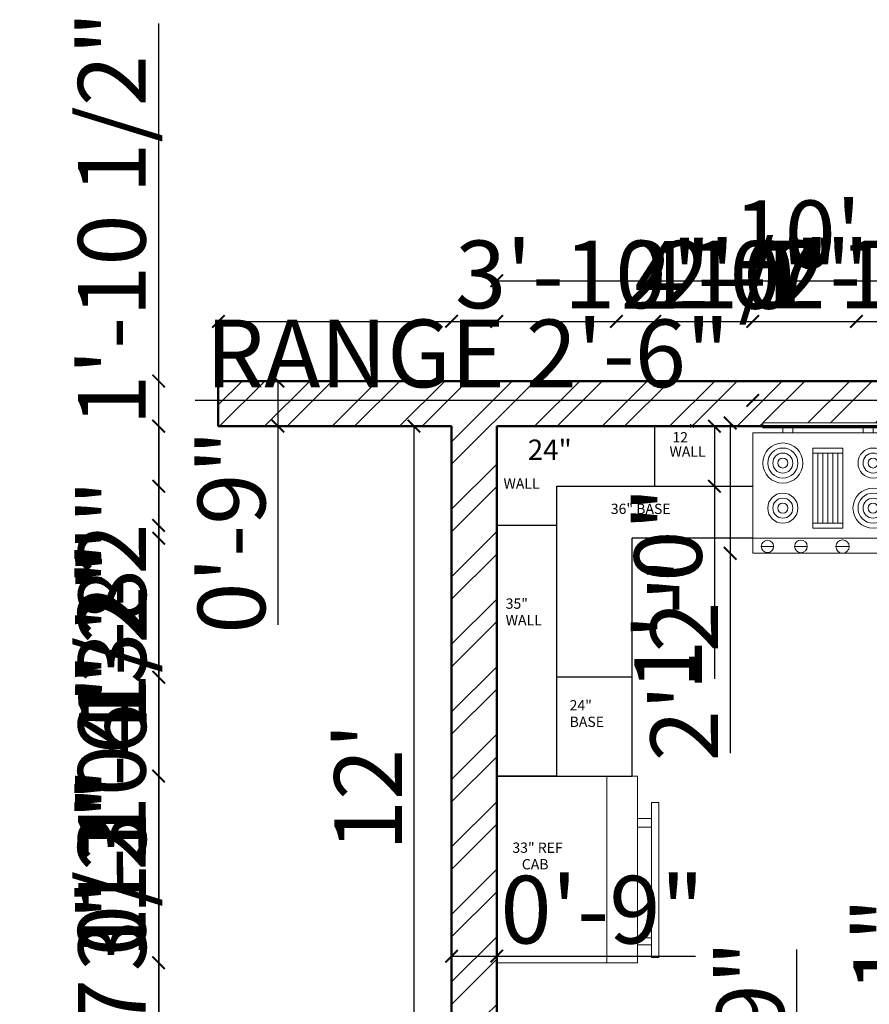
# Model space of a CAD drawing. Units: inches. Extents: x 1736 to 2023, y 1717 to 2014.
# Tile 2 of 3: x 1736 to 1906, y 1818 to 2014. Entities that reach past the tile are written whole.
import ezdxf

# ---------------------------------------------------------------- set-up
doc = ezdxf.new("R2010")
doc.units = ezdxf.units.IN
for name, color, linetype, lineweight in [('A-ANNO-DIMS', 2, 'Continuous', 18), ('A-ANNO-TEXT', 3, 'Continuous', 18), ('A-EQPM', 9, 'Continuous', 18), ('A-FLOR-CASE', 8, 'Continuous', 25), ('A-WALL', 7, 'Continuous', 50), ('A-WALL-PATT', 8, 'Continuous', 13)]:
    doc.layers.add(name, color=color, linetype=linetype, lineweight=lineweight)
doc.styles.get("Standard").update_dxf_attribs({"font": 'arial.ttf'})
doc.dimstyles.new('ISO-25', dxfattribs={"dimtxt": 13.5, "dimasz": 2.5, "dimexe": 1.25, "dimexo": 0.625, "dimtad": 1, "dimdec": 0, "dimlunit": 4, "dimtxsty": 'Standard', "dimblk": 'ARCHTICK', "dimcen": 2.5, "dimse1": 1, "dimse2": 1, "dimclrd": 2, "dimclrt": 4, "dimadec": 0, "dimazin": 0, "dimtfac": 1, "dimtdec": 0, "dimtmove": 0, "dimatfit": 3, "dimfxl": 1, "dimarcsym": 0})

# ---------------------------------------------------------------- blocks, each defined once
blk = doc.blocks.new('Range-Oven - 30 in top')
for p, q in [((0, -3), (30, -3)), ((12, -6), (18, -6)), ((13, -20), (13, -6)), ((14, -6), (14, -20)), ((15, -20), (15, -6)), ((16, -6), (16, -20)), ((17, -20), (17, -6)), ((18, -20), (12, -20)), ((6, -24), (6, -25)), ((8, -25), (8, -24)), ((22, -25), (22, -24)), ((24, -24), (24, -25))]:
    blk.add_line(p, q)
for points in [[(0, -24), (0, 0), (30, 0), (30, -24)], [(12, -21), (12, -5), (18, -5), (18, -21)], [(2, -26), (2, -25), (28, -25), (28, -26)]]:
    blk.add_lwpolyline(points, close=True)
for centre, radius in [((6, -9), 4), ((6, -9), 3), ((6, -9), 2), ((24, -9), 3), ((24, -9), 2), ((6, -9), 1), ((24, -9), 1), ((6, -18), 3), ((24, -18), 4), ((24, -18), 3), ((6, -18), 2), ((6, -18), 1), ((24, -18), 2), ((24, -18), 1)]:
    blk.add_circle(centre, radius)
blk = doc.blocks.new('_ArchTick')
at = {"color": 0, "linetype": 'ByBlock', "const_width": 0.15}
blk.add_lwpolyline([(-0.5, -0.5), (0.5, 0.5)], dxfattribs=at)
blk = doc.blocks.new('*D7')
at = {"layer": 'A-ANNO-DIMS', "color": 0, "lineweight": -2, "transparency": 16777216}
blk.add_line((1831.43, 1962.29), (1951.43, 1962.29), dxfattribs=at)
at = {"layer": 'Defpoints', "color": 0, "transparency": 16777216}
for p in [(1951.43, 1962.29), (1831.43, 1933.29), (1951.43, 1933.29)]:
    blk.add_point(p, dxfattribs=at)
at = {"layer": 'A-ANNO-DIMS', "color": 0, "lineweight": -2, "transparency": 16777216, "xscale": 2.5, "yscale": 2.5, "zscale": 2.5, "rotation": 180}
blk.add_blockref('_ArchTick', (1831.43, 1962.29), dxfattribs=at)
at = {"layer": 'A-ANNO-DIMS', "color": 0, "lineweight": -2, "transparency": 16777216, "xscale": 2.5, "yscale": 2.5, "zscale": 2.5}
blk.add_blockref('_ArchTick', (1951.43, 1962.29), dxfattribs=at)
at = {"layer": 'A-ANNO-DIMS', "color": 0, "transparency": 16777216, "insert": (1891.43, 1969.8), "char_height": 13.5, "attachment_point": 5}
blk.add_mtext("10'", dxfattribs=at)
blk = doc.blocks.new('*D8')
at = {"layer": 'A-ANNO-DIMS', "color": 0, "lineweight": -2, "transparency": 16777216}
blk.add_line((1814.91, 1933.29), (1814.91, 1789.29), dxfattribs=at)
at = {"layer": 'Defpoints', "color": 0, "transparency": 16777216}
for p in [(1822.43, 1933.29), (1814.91, 1789.29), (1822.43, 1789.29)]:
    blk.add_point(p, dxfattribs=at)
at = {"layer": 'A-ANNO-DIMS', "color": 0, "lineweight": -2, "transparency": 16777216, "xscale": 2.5, "yscale": 2.5, "zscale": 2.5}
for p, rotation in [((1814.91, 1933.29), 90), ((1814.91, 1789.29), 270)]:
    blk.add_blockref('_ArchTick', p, dxfattribs=dict(at, rotation=rotation))
at = {"layer": 'A-ANNO-DIMS', "color": 0, "transparency": 16777216, "insert": (1807.51, 1861.29), "char_height": 13.5, "attachment_point": 5, "rotation": 90}
blk.add_mtext("12'", dxfattribs=at)
blk = doc.blocks.new('*D9')
at = {"layer": 'A-ANNO-DIMS', "color": 2, "lineweight": -2, "transparency": 16777216}
for p, q in [((1882.52, 1938.43), (1771.27, 1938.43)), ((1912.52, 1938.43), (1882.52, 1938.43))]:
    blk.add_line(p, q, dxfattribs=at)
at = {"layer": 'Defpoints', "color": 0, "transparency": 16777216}
for p in [(1882.52, 1938.43), (1882.52, 1933.93), (1912.52, 1933.93)]:
    blk.add_point(p, dxfattribs=at)
at = {"layer": 'A-ANNO-DIMS', "color": 2, "lineweight": -2, "transparency": 16777216, "xscale": 2.5, "yscale": 2.5, "zscale": 2.5, "rotation": 180}
blk.add_blockref('_ArchTick', (1882.52, 1938.43), dxfattribs=at)
at = {"layer": 'A-ANNO-DIMS', "color": 2, "lineweight": -2, "transparency": 16777216, "xscale": 2.5, "yscale": 2.5, "zscale": 2.5}
blk.add_blockref('_ArchTick', (1912.52, 1938.43), dxfattribs=at)
at = {"layer": 'A-ANNO-DIMS', "color": 4, "transparency": 16777216, "insert": (1825.64, 1946.04), "char_height": 13.5, "attachment_point": 5}
blk.add_mtext('RANGE 2\'-6"', dxfattribs=at)
blk = doc.blocks.new('*D10')
at = {"layer": 'A-ANNO-DIMS', "color": 2, "lineweight": -2, "transparency": 16777216}
for p, q in [((1878.02, 1933.93), (1878.02, 1907.93)), ((1878.02, 1907.93), (1878.02, 1868.07))]:
    blk.add_line(p, q, dxfattribs=at)
at = {"layer": 'Defpoints', "color": 0, "transparency": 16777216}
for p in [(1882.52, 1933.93), (1878.02, 1907.93), (1882.52, 1907.93)]:
    blk.add_point(p, dxfattribs=at)
at = {"layer": 'A-ANNO-DIMS', "color": 2, "lineweight": -2, "transparency": 16777216, "xscale": 2.5, "yscale": 2.5, "zscale": 2.5}
for p, rotation in [((1878.02, 1933.93), 90), ((1878.02, 1907.93), 270)]:
    blk.add_blockref('_ArchTick', p, dxfattribs=dict(at, rotation=rotation))
at = {"layer": 'A-ANNO-DIMS', "color": 4, "transparency": 16777216, "insert": (1870.61, 1886.75), "char_height": 13.5, "attachment_point": 5, "rotation": 90}
blk.add_mtext('2\'-2"', dxfattribs=at)
blk = doc.blocks.new('*D14')
at = {"layer": 'A-ANNO-DIMS', "color": 2, "lineweight": -2, "transparency": 16777216}
blk.add_line((1763.99, 1780.29), (1763.99, 1942.29), dxfattribs=at)
at = {"layer": 'Defpoints', "color": 0, "transparency": 16777216}
for p in [(1763.99, 1942.29), (1775.89, 1942.29), (1775.89, 1780.29)]:
    blk.add_point(p, dxfattribs=at)
at = {"layer": 'A-ANNO-DIMS', "color": 2, "lineweight": -2, "transparency": 16777216, "xscale": 2.5, "yscale": 2.5, "zscale": 2.5}
for p, rotation in [((1763.99, 1942.29), 90), ((1763.99, 1780.29), 270)]:
    blk.add_blockref('_ArchTick', p, dxfattribs=dict(at, rotation=rotation))
at = {"layer": 'A-ANNO-DIMS', "color": 4, "transparency": 16777216, "insert": (1756.47, 1861.29), "char_height": 13.5, "attachment_point": 5, "rotation": 90}
blk.add_mtext('13\'-6"', dxfattribs=at)
blk = doc.blocks.new('*D15')
at = {"layer": 'A-ANNO-DIMS', "color": 2, "lineweight": -2, "transparency": 16777216}
for p, q in [((1787.79, 1942.29), (1787.79, 1933.29)), ((1787.79, 1933.29), (1787.79, 1893.65))]:
    blk.add_line(p, q, dxfattribs=at)
at = {"layer": 'Defpoints', "color": 0, "transparency": 16777216}
for p in [(1775.89, 1942.29), (1775.89, 1933.29), (1787.79, 1933.29)]:
    blk.add_point(p, dxfattribs=at)
at = {"layer": 'A-ANNO-DIMS', "color": 2, "lineweight": -2, "transparency": 16777216, "xscale": 2.5, "yscale": 2.5, "zscale": 2.5}
for p, rotation in [((1787.79, 1942.29), 90), ((1787.79, 1933.29), 270)]:
    blk.add_blockref('_ArchTick', p, dxfattribs=dict(at, rotation=rotation))
at = {"layer": 'A-ANNO-DIMS', "color": 4, "transparency": 16777216, "insert": (1780.27, 1912.22), "char_height": 13.5, "attachment_point": 5, "rotation": 90}
blk.add_mtext('0\'-9"', dxfattribs=at)
blk = doc.blocks.new('*D17')
at = {"layer": 'A-ANNO-DIMS', "color": 2, "lineweight": -2, "transparency": 16777216}
for p, q in [((1891.31, 1789.29), (1891.31, 1828.92)), ((1891.31, 1780.29), (1891.31, 1789.29))]:
    blk.add_line(p, q, dxfattribs=at)
at = {"layer": 'Defpoints', "color": 0, "transparency": 16777216}
for p in [(1891.31, 1789.29), (1903.21, 1789.29), (1903.21, 1780.29)]:
    blk.add_point(p, dxfattribs=at)
at = {"layer": 'A-ANNO-DIMS', "color": 2, "lineweight": -2, "transparency": 16777216, "xscale": 2.5, "yscale": 2.5, "zscale": 2.5}
for p, rotation in [((1891.31, 1789.29), 90), ((1891.31, 1780.29), 270)]:
    blk.add_blockref('_ArchTick', p, dxfattribs=dict(at, rotation=rotation))
at = {"layer": 'A-ANNO-DIMS', "color": 4, "transparency": 16777216, "insert": (1883.79, 1810.35), "char_height": 13.5, "attachment_point": 5, "rotation": 90}
blk.add_mtext('0\'-9"', dxfattribs=at)
blk = doc.blocks.new('*D18')
at = {"layer": 'A-ANNO-DIMS', "color": 2, "lineweight": -2, "transparency": 16777216}
for p, q in [((1822.43, 1827.58), (1831.43, 1827.58)), ((1831.43, 1827.58), (1871.07, 1827.58))]:
    blk.add_line(p, q, dxfattribs=at)
at = {"layer": 'Defpoints', "color": 0, "transparency": 16777216}
for p in [(1831.43, 1827.58), (1822.43, 1815.68), (1831.43, 1815.68)]:
    blk.add_point(p, dxfattribs=at)
at = {"layer": 'A-ANNO-DIMS', "color": 2, "lineweight": -2, "transparency": 16777216, "xscale": 2.5, "yscale": 2.5, "zscale": 2.5, "rotation": 180}
blk.add_blockref('_ArchTick', (1822.43, 1827.58), dxfattribs=at)
at = {"layer": 'A-ANNO-DIMS', "color": 2, "lineweight": -2, "transparency": 16777216, "xscale": 2.5, "yscale": 2.5, "zscale": 2.5}
blk.add_blockref('_ArchTick', (1831.43, 1827.58), dxfattribs=at)
at = {"layer": 'A-ANNO-DIMS', "color": 4, "transparency": 16777216, "insert": (1852.5, 1835.1), "char_height": 13.5, "attachment_point": 5}
blk.add_mtext('0\'-9"', dxfattribs=at)
blk = doc.blocks.new('*D19')
at = {"layer": 'A-ANNO-DIMS', "color": 2, "lineweight": -2, "transparency": 16777216}
for p, q in [((1775.89, 1954.19), (1822.43, 1954.19)), ((1822.43, 1954.19), (1904.01, 1954.19))]:
    blk.add_line(p, q, dxfattribs=at)
at = {"layer": 'Defpoints', "color": 0, "transparency": 16777216}
for p in [(1822.43, 1954.19), (1775.89, 1942.29), (1822.43, 1933.29)]:
    blk.add_point(p, dxfattribs=at)
at = {"layer": 'A-ANNO-DIMS', "color": 2, "lineweight": -2, "transparency": 16777216, "xscale": 2.5, "yscale": 2.5, "zscale": 2.5, "rotation": 180}
blk.add_blockref('_ArchTick', (1775.89, 1954.19), dxfattribs=at)
at = {"layer": 'A-ANNO-DIMS', "color": 2, "lineweight": -2, "transparency": 16777216, "xscale": 2.5, "yscale": 2.5, "zscale": 2.5}
blk.add_blockref('_ArchTick', (1822.43, 1954.19), dxfattribs=at)
at = {"layer": 'A-ANNO-DIMS', "color": 4, "transparency": 16777216, "insert": (1864.47, 1961.8), "char_height": 13.5, "attachment_point": 5}
blk.add_mtext('3\'-10 1/2"', dxfattribs=at)
blk = doc.blocks.new('*D22')
at = {"layer": 'A-ANNO-DIMS', "color": 2, "lineweight": -2, "transparency": 16777216}
for p, q in [((1831.43, 1954.19), (1855.31, 1954.19)), ((1855.31, 1954.19), (1895.17, 1954.19))]:
    blk.add_line(p, q, dxfattribs=at)
at = {"layer": 'Defpoints', "color": 0, "transparency": 16777216}
for p in [(1855.31, 1954.19), (1831.43, 1789.29), (1855.31, 1789.29)]:
    blk.add_point(p, dxfattribs=at)
at = {"layer": 'A-ANNO-DIMS', "color": 2, "lineweight": -2, "transparency": 16777216, "xscale": 2.5, "yscale": 2.5, "zscale": 2.5, "rotation": 180}
blk.add_blockref('_ArchTick', (1831.43, 1954.19), dxfattribs=at)
at = {"layer": 'A-ANNO-DIMS', "color": 2, "lineweight": -2, "transparency": 16777216, "xscale": 2.5, "yscale": 2.5, "zscale": 2.5}
blk.add_blockref('_ArchTick', (1855.31, 1954.19), dxfattribs=at)
at = {"layer": 'A-ANNO-DIMS', "color": 4, "transparency": 16777216, "insert": (1876.49, 1961.7), "char_height": 13.5, "attachment_point": 5}
blk.add_mtext('2\'-0"', dxfattribs=at)
blk = doc.blocks.new('*D23')
at = {"layer": 'A-ANNO-DIMS', "color": 2, "lineweight": -2, "transparency": 16777216}
blk.add_line((1855.31, 1954.19), (1903.21, 1954.19), dxfattribs=at)
at = {"layer": 'Defpoints', "color": 0, "transparency": 16777216}
for p in [(1903.21, 1954.19), (1855.31, 1789.29), (1903.21, 1789.29)]:
    blk.add_point(p, dxfattribs=at)
at = {"layer": 'A-ANNO-DIMS', "color": 2, "lineweight": -2, "transparency": 16777216, "xscale": 2.5, "yscale": 2.5, "zscale": 2.5, "rotation": 180}
blk.add_blockref('_ArchTick', (1855.31, 1954.19), dxfattribs=at)
at = {"layer": 'A-ANNO-DIMS', "color": 2, "lineweight": -2, "transparency": 16777216, "xscale": 2.5, "yscale": 2.5, "zscale": 2.5}
blk.add_blockref('_ArchTick', (1903.21, 1954.19), dxfattribs=at)
at = {"layer": 'A-ANNO-DIMS', "color": 4, "transparency": 16777216, "insert": (1879.26, 1961.7), "char_height": 13.5, "attachment_point": 5}
blk.add_mtext('4\'-0"', dxfattribs=at)
blk = doc.blocks.new('*D28')
at = {"layer": 'A-ANNO-DIMS', "color": 2, "lineweight": -2, "transparency": 16777216}
for p, q in [((1918.58, 1795.35), (1918.58, 1837.48)), ((1918.58, 1794.21), (1918.58, 1795.35)), ((1918.58, 1794.21), (1918.58, 1791.71))]:
    blk.add_line(p, q, dxfattribs=at)
at = {"layer": 'Defpoints', "color": 0, "transparency": 16777216}
for p in [(1918.58, 1795.35), (1930.48, 1795.35), (1930.48, 1794.21)]:
    blk.add_point(p, dxfattribs=at)
at = {"layer": 'A-ANNO-DIMS', "color": 2, "lineweight": -2, "transparency": 16777216, "xscale": 2.5, "yscale": 2.5, "zscale": 2.5}
for p, rotation in [((1918.58, 1795.35), 270), ((1918.58, 1794.21), 90)]:
    blk.add_blockref('_ArchTick', p, dxfattribs=dict(at, rotation=rotation))
at = {"layer": 'A-ANNO-DIMS', "color": 4, "transparency": 16777216, "insert": (1911.06, 1818.91), "char_height": 13.5, "attachment_point": 5, "rotation": 90}
blk.add_mtext('0\'-1"', dxfattribs=at)
blk = doc.blocks.new('*D29')
at = {"layer": 'A-ANNO-DIMS', "color": 2, "lineweight": -2, "transparency": 16777216}
for p, q in [((1874.87, 1933.29), (1874.87, 1921.29)), ((1874.87, 1921.29), (1874.87, 1882.92))]:
    blk.add_line(p, q, dxfattribs=at)
at = {"layer": 'Defpoints', "color": 0, "transparency": 16777216}
for p in [(1862.97, 1933.29), (1862.97, 1921.29), (1874.87, 1921.29)]:
    blk.add_point(p, dxfattribs=at)
at = {"layer": 'A-ANNO-DIMS', "color": 2, "lineweight": -2, "transparency": 16777216, "xscale": 2.5, "yscale": 2.5, "zscale": 2.5}
for p, rotation in [((1874.87, 1933.29), 90), ((1874.87, 1921.29), 270)]:
    blk.add_blockref('_ArchTick', p, dxfattribs=dict(at, rotation=rotation))
at = {"layer": 'A-ANNO-DIMS', "color": 4, "transparency": 16777216, "insert": (1867.36, 1900.85), "char_height": 13.5, "attachment_point": 5, "rotation": 90}
blk.add_mtext('1\'-0"', dxfattribs=at)
blk = doc.blocks.new('*D30')
at = {"layer": 'A-ANNO-DIMS', "color": 2, "lineweight": -2, "transparency": 16777216}
for p, q in [((1763.99, 1933.29), (1763.99, 2013.6)), ((1763.99, 1910.93), (1763.99, 1933.29))]:
    blk.add_line(p, q, dxfattribs=at)
at = {"layer": 'Defpoints', "color": 0, "transparency": 16777216}
for p in [(1763.99, 1933.29), (1951.43, 1933.29), (1934.43, 1910.93)]:
    blk.add_point(p, dxfattribs=at)
at = {"layer": 'A-ANNO-DIMS', "color": 2, "lineweight": -2, "transparency": 16777216, "xscale": 2.5, "yscale": 2.5, "zscale": 2.5}
for p, rotation in [((1763.99, 1933.29), 90), ((1763.99, 1910.93), 270)]:
    blk.add_blockref('_ArchTick', p, dxfattribs=dict(at, rotation=rotation))
at = {"layer": 'A-ANNO-DIMS', "color": 4, "transparency": 16777216, "insert": (1756.39, 1974.69), "char_height": 13.5, "attachment_point": 5, "rotation": 90}
blk.add_mtext('1\'-10 1/2"', dxfattribs=at)
blk = doc.blocks.new('*D32')
at = {"layer": 'A-ANNO-DIMS', "color": 2, "lineweight": -2, "transparency": 16777216}
for p, q in [((1831.43, 1732.64), (1843.43, 1732.64)), ((1843.43, 1732.64), (1881.8, 1732.64))]:
    blk.add_line(p, q, dxfattribs=at)
at = {"layer": 'Defpoints', "color": 0, "transparency": 16777216}
for p in [(1831.43, 1913.5), (1843.43, 1913.5), (1843.43, 1732.64)]:
    blk.add_point(p, dxfattribs=at)
at = {"layer": 'A-ANNO-DIMS', "color": 2, "lineweight": -2, "transparency": 16777216, "xscale": 2.5, "yscale": 2.5, "zscale": 2.5, "rotation": 180}
blk.add_blockref('_ArchTick', (1831.43, 1732.64), dxfattribs=at)
at = {"layer": 'A-ANNO-DIMS', "color": 2, "lineweight": -2, "transparency": 16777216, "xscale": 2.5, "yscale": 2.5, "zscale": 2.5}
blk.add_blockref('_ArchTick', (1843.43, 1732.64), dxfattribs=at)
at = {"layer": 'A-ANNO-DIMS', "color": 4, "transparency": 16777216, "insert": (1863.87, 1740.16), "char_height": 13.5, "attachment_point": 5}
blk.add_mtext('1\'-0"', dxfattribs=at)
blk = doc.blocks.new('*D33')
at = {"layer": 'A-ANNO-DIMS', "color": 2, "lineweight": -2, "transparency": 16777216}
for p, q in [((1831.43, 1732.64), (1858.43, 1732.64)), ((1858.43, 1732.64), (1898.3, 1732.64))]:
    blk.add_line(p, q, dxfattribs=at)
at = {"layer": 'Defpoints', "color": 0, "transparency": 16777216}
for p in [(1831.43, 1863.49), (1858.43, 1863.49), (1858.43, 1732.64)]:
    blk.add_point(p, dxfattribs=at)
at = {"layer": 'A-ANNO-DIMS', "color": 2, "lineweight": -2, "transparency": 16777216, "xscale": 2.5, "yscale": 2.5, "zscale": 2.5, "rotation": 180}
blk.add_blockref('_ArchTick', (1831.43, 1732.64), dxfattribs=at)
at = {"layer": 'A-ANNO-DIMS', "color": 2, "lineweight": -2, "transparency": 16777216, "xscale": 2.5, "yscale": 2.5, "zscale": 2.5}
blk.add_blockref('_ArchTick', (1858.43, 1732.64), dxfattribs=at)
at = {"layer": 'A-ANNO-DIMS', "color": 4, "transparency": 16777216, "insert": (1879.62, 1740.16), "char_height": 13.5, "attachment_point": 5}
blk.add_mtext('2\'-3"', dxfattribs=at)
blk = doc.blocks.new('*D34')
at = {"layer": 'A-ANNO-DIMS', "color": 2, "lineweight": -2, "transparency": 16777216}
for p, q in [((1831.43, 1954.19), (1862.97, 1954.19)), ((1862.97, 1954.19), (1934.3, 1954.19))]:
    blk.add_line(p, q, dxfattribs=at)
at = {"layer": 'Defpoints', "color": 0, "transparency": 16777216}
for p in [(1862.97, 1954.19), (1831.43, 1933.29), (1862.97, 1933.29)]:
    blk.add_point(p, dxfattribs=at)
at = {"layer": 'A-ANNO-DIMS', "color": 2, "lineweight": -2, "transparency": 16777216, "xscale": 2.5, "yscale": 2.5, "zscale": 2.5, "rotation": 180}
blk.add_blockref('_ArchTick', (1831.43, 1954.19), dxfattribs=at)
at = {"layer": 'A-ANNO-DIMS', "color": 2, "lineweight": -2, "transparency": 16777216, "xscale": 2.5, "yscale": 2.5, "zscale": 2.5}
blk.add_blockref('_ArchTick', (1862.97, 1954.19), dxfattribs=at)
at = {"layer": 'A-ANNO-DIMS', "color": 4, "transparency": 16777216, "insert": (1899.89, 1961.79), "char_height": 13.5, "attachment_point": 5}
blk.add_mtext('2\'-7 1/2"', dxfattribs=at)
blk = doc.blocks.new('*D35')
at = {"layer": 'A-ANNO-DIMS', "color": 2, "lineweight": -2, "transparency": 16777216}
for p, q in [((1862.97, 1954.19), (1882.52, 1954.19)), ((1882.52, 1954.19), (1952.34, 1954.19))]:
    blk.add_line(p, q, dxfattribs=at)
at = {"layer": 'Defpoints', "color": 0, "transparency": 16777216}
for p in [(1882.52, 1954.19), (1862.97, 1921.29), (1882.52, 1921.29)]:
    blk.add_point(p, dxfattribs=at)
at = {"layer": 'A-ANNO-DIMS', "color": 2, "lineweight": -2, "transparency": 16777216, "xscale": 2.5, "yscale": 2.5, "zscale": 2.5, "rotation": 180}
blk.add_blockref('_ArchTick', (1862.97, 1954.19), dxfattribs=at)
at = {"layer": 'A-ANNO-DIMS', "color": 2, "lineweight": -2, "transparency": 16777216, "xscale": 2.5, "yscale": 2.5, "zscale": 2.5}
blk.add_blockref('_ArchTick', (1882.52, 1954.19), dxfattribs=at)
at = {"layer": 'A-ANNO-DIMS', "color": 4, "transparency": 16777216, "insert": (1918.68, 1961.79), "char_height": 13.5, "attachment_point": 5}
blk.add_mtext('1\'-7 1/2"', dxfattribs=at)
blk = doc.blocks.new('*D38')
at = {"layer": 'A-ANNO-DIMS', "color": 2, "lineweight": -2, "transparency": 16777216}
for p, q in [((1763.99, 1933.29), (1763.99, 1913.5)), ((1763.99, 1913.5), (1763.99, 1875.14))]:
    blk.add_line(p, q, dxfattribs=at)
at = {"layer": 'Defpoints', "color": 0, "transparency": 16777216}
for p in [(1831.43, 1933.29), (1763.99, 1913.5), (1831.43, 1913.5)]:
    blk.add_point(p, dxfattribs=at)
at = {"layer": 'A-ANNO-DIMS', "color": 2, "lineweight": -2, "transparency": 16777216, "xscale": 2.5, "yscale": 2.5, "zscale": 2.5}
for p, rotation in [((1763.99, 1933.29), 90), ((1763.99, 1913.5), 270)]:
    blk.add_blockref('_ArchTick', p, dxfattribs=dict(at, rotation=rotation))
at = {"layer": 'A-ANNO-DIMS', "color": 4, "transparency": 16777216, "insert": (1756.47, 1893.07), "char_height": 13.5, "attachment_point": 5, "rotation": 90}
blk.add_mtext('1\'-8"', dxfattribs=at)
blk = doc.blocks.new('*D39')
at = {"layer": 'A-ANNO-DIMS', "color": 2, "lineweight": -2, "transparency": 16777216}
blk.add_line((1763.99, 1913.5), (1763.99, 1863.49), dxfattribs=at)
at = {"layer": 'Defpoints', "color": 0, "transparency": 16777216}
for p in [(1831.43, 1913.5), (1763.99, 1863.49), (1831.43, 1863.49)]:
    blk.add_point(p, dxfattribs=at)
at = {"layer": 'A-ANNO-DIMS', "color": 2, "lineweight": -2, "transparency": 16777216, "xscale": 2.5, "yscale": 2.5, "zscale": 2.5}
for p, rotation in [((1763.99, 1913.5), 90), ((1763.99, 1863.49), 270)]:
    blk.add_blockref('_ArchTick', p, dxfattribs=dict(at, rotation=rotation))
at = {"layer": 'A-ANNO-DIMS', "color": 4, "transparency": 16777216, "insert": (1756.59, 1888.5), "char_height": 13.5, "attachment_point": 5, "rotation": 90}
blk.add_mtext('4\'-2"', dxfattribs=at)
blk = doc.blocks.new('*D40')
at = {"layer": 'A-ANNO-DIMS', "color": 2, "lineweight": -2, "transparency": 16777216}
blk.add_line((1763.99, 1863.49), (1763.99, 1826.26), dxfattribs=at)
at = {"layer": 'Defpoints', "color": 0, "transparency": 16777216}
for p in [(1831.43, 1863.49), (1763.99, 1826.26), (1831.43, 1826.26)]:
    blk.add_point(p, dxfattribs=at)
at = {"layer": 'A-ANNO-DIMS', "color": 2, "lineweight": -2, "transparency": 16777216, "xscale": 2.5, "yscale": 2.5, "zscale": 2.5}
for p, rotation in [((1763.99, 1863.49), 90), ((1763.99, 1826.26), 270)]:
    blk.add_blockref('_ArchTick', p, dxfattribs=dict(at, rotation=rotation))
at = {"layer": 'A-ANNO-DIMS', "color": 4, "transparency": 16777216, "insert": (1756.47, 1844.88), "char_height": 13.5, "attachment_point": 5, "rotation": 90}
blk.add_mtext('3\'-1"', dxfattribs=at)
blk = doc.blocks.new('*D41')
at = {"layer": 'A-ANNO-DIMS', "color": 2, "lineweight": -2, "transparency": 16777216}
blk.add_line((1763.99, 1921.29), (1763.99, 1883.21), dxfattribs=at)
at = {"layer": 'Defpoints', "color": 0, "transparency": 16777216}
for p in [(1843.43, 1921.29), (1763.99, 1883.21), (1843.43, 1883.21)]:
    blk.add_point(p, dxfattribs=at)
at = {"layer": 'A-ANNO-DIMS', "color": 2, "lineweight": -2, "transparency": 16777216, "xscale": 2.5, "yscale": 2.5, "zscale": 2.5}
for p, rotation in [((1763.99, 1921.29), 90), ((1763.99, 1883.21), 270)]:
    blk.add_blockref('_ArchTick', p, dxfattribs=dict(at, rotation=rotation))
at = {"layer": 'A-ANNO-DIMS', "color": 4, "transparency": 16777216, "insert": (1756.47, 1902.25), "char_height": 13.5, "attachment_point": 5, "rotation": 90}
blk.add_mtext('3\'-2"', dxfattribs=at)
blk = doc.blocks.new('*D42')
at = {"layer": 'A-ANNO-DIMS', "color": 2, "lineweight": -2, "transparency": 16777216}
for p, q in [((1763.99, 1883.21), (1763.99, 1863.49)), ((1763.99, 1863.49), (1763.99, 1793.67))]:
    blk.add_line(p, q, dxfattribs=at)
at = {"layer": 'Defpoints', "color": 0, "transparency": 16777216}
for p in [(1843.43, 1883.21), (1763.99, 1863.49), (1843.43, 1863.49)]:
    blk.add_point(p, dxfattribs=at)
at = {"layer": 'A-ANNO-DIMS', "color": 2, "lineweight": -2, "transparency": 16777216, "xscale": 2.5, "yscale": 2.5, "zscale": 2.5}
for p, rotation in [((1763.99, 1883.21), 90), ((1763.99, 1863.49), 270)]:
    blk.add_blockref('_ArchTick', p, dxfattribs=dict(at, rotation=rotation))
at = {"layer": 'A-ANNO-DIMS', "color": 4, "transparency": 16777216, "insert": (1756.39, 1827.33), "char_height": 13.5, "attachment_point": 5, "rotation": 90}
blk.add_mtext('1\'-7 1/2"', dxfattribs=at)
blk = doc.blocks.new('*D43')
at = {"layer": 'A-ANNO-DIMS', "color": 2, "lineweight": -2, "transparency": 16777216}
blk.add_line((1843.43, 1732.64), (1882.52, 1732.64), dxfattribs=at)
at = {"layer": 'Defpoints', "color": 0, "transparency": 16777216}
for p in [(1843.43, 1921.29), (1882.52, 1921.29), (1882.52, 1732.64)]:
    blk.add_point(p, dxfattribs=at)
at = {"layer": 'A-ANNO-DIMS', "color": 2, "lineweight": -2, "transparency": 16777216, "xscale": 2.5, "yscale": 2.5, "zscale": 2.5, "rotation": 180}
blk.add_blockref('_ArchTick', (1843.43, 1732.64), dxfattribs=at)
at = {"layer": 'A-ANNO-DIMS', "color": 2, "lineweight": -2, "transparency": 16777216, "xscale": 2.5, "yscale": 2.5, "zscale": 2.5}
blk.add_blockref('_ArchTick', (1882.52, 1732.64), dxfattribs=at)
at = {"layer": 'A-ANNO-DIMS', "color": 4, "transparency": 16777216, "insert": (1862.97, 1740.16), "char_height": 13.5, "attachment_point": 5}
blk.add_mtext('3\'-3"', dxfattribs=at)
blk = doc.blocks.new('*D44')
at = {"layer": 'A-ANNO-DIMS', "color": 2, "lineweight": -2, "transparency": 16777216}
for p, q in [((1763.99, 1921.29), (1763.99, 1910.93)), ((1763.99, 1910.93), (1763.99, 1829.35))]:
    blk.add_line(p, q, dxfattribs=at)
at = {"layer": 'Defpoints', "color": 0, "transparency": 16777216}
for p in [(1862.97, 1921.29), (1763.99, 1910.93), (1858.43, 1910.93)]:
    blk.add_point(p, dxfattribs=at)
at = {"layer": 'A-ANNO-DIMS', "color": 2, "lineweight": -2, "transparency": 16777216, "xscale": 2.5, "yscale": 2.5, "zscale": 2.5}
for p, rotation in [((1763.99, 1921.29), 90), ((1763.99, 1910.93), 270)]:
    blk.add_blockref('_ArchTick', p, dxfattribs=dict(at, rotation=rotation))
at = {"layer": 'A-ANNO-DIMS', "color": 4, "transparency": 16777216, "insert": (1756.39, 1868.89), "char_height": 13.5, "attachment_point": 5, "rotation": 90}
blk.add_mtext('0\'-10 1/2"', dxfattribs=at)

msp = doc.modelspace()

# ---------------------------------------------------------------- hatches: boundary and pattern name
at = {"layer": 'A-WALL-PATT'}
h = msp.add_hatch(dxfattribs=at)
h.set_pattern_fill('ANSI32', color=256)
h.paths.add_polyline_path([(1831.43, 1933.29), (1884.52, 1933.29), (1884.52, 1933.93), (1910.52, 1933.93), (1910.52, 1933.29), (1951.43, 1933.29), (1951.43, 1911.39), (1960.43, 1911.39), (1960.43, 1942.29), (1822.43, 1942.29), (1775.89, 1942.29), (1775.89, 1933.29), (1822.43, 1933.29), (1822.43, 1815.68), (1831.43, 1815.68)])
h.paths.add_polyline_path([(1960.43, 1848.88), (1951.43, 1848.88), (1951.43, 1819.75, -0.049233), (1956.53, 1820.25), (1960.43, 1820.25)], flags=17)
h.paths.add_polyline_path([(1960.43, 1794.21), (1956.53, 1794.21), (1951.43, 1794.21), (1951.43, 1789.29), (1903.21, 1789.29), (1903.21, 1780.29), (1960.43, 1780.29)])
h.paths.add_polyline_path([(1855.31, 1789.29), (1831.43, 1789.29), (1831.43, 1793.62), (1822.43, 1793.62), (1822.43, 1789.29), (1775.89, 1789.29), (1775.89, 1780.29), (1822.43, 1780.29), (1855.31, 1780.29)])

# ---------------------------------------------------------------- linework, layer by layer
at = {"layer": 'A-EQPM'}
for p, q in [((1884.23, 1909.31), (1886.66, 1909.31)), ((1890.86, 1909.31), (1893.38, 1909.31)), ((1899.11, 1909.27), (1901.78, 1909.27)), ((1853.39, 1863.49), (1853.39, 1826.26)), ((1858.43, 1863.49), (1859.53, 1863.49)), ((1859.53, 1863.49), (1859.53, 1826.26)), ((1862.34, 1855), (1859.53, 1855)), ((1862.34, 1853.28), (1859.53, 1853.28)), ((1862.34, 1831.21), (1859.53, 1831.21)), ((1862.34, 1829.82), (1859.53, 1829.82)), ((1859.53, 1826.26), (1831.43, 1826.26))]:
    msp.add_line(p, q, dxfattribs=at)
msp.add_lwpolyline([(1862.34, 1858.23), (1863.78, 1858.23), (1863.78, 1827.31), (1862.34, 1827.31)], close=True, dxfattribs=at)
for centre, radius in [((1885.45, 1909.31), 1.22), ((1892.12, 1909.31), 1.26), ((1900.44, 1909.27), 1.33)]:
    msp.add_circle(centre, radius, dxfattribs=at)
at = {"layer": 'A-FLOR-CASE'}
for p, q in [((1862.97, 1921.29), (1862.97, 1933.29)), ((1843.43, 1863.49), (1843.43, 1921.29)), ((1843.43, 1921.29), (1882.52, 1921.29)), ((1843.43, 1913.5), (1831.43, 1913.5)), ((1858.43, 1863.49), (1858.43, 1910.93)), ((1882.52, 1910.93), (1858.43, 1910.93)), ((1858.43, 1883.21), (1843.43, 1883.21)), ((1843.43, 1863.49), (1831.43, 1863.49)), ((1831.43, 1863.49), (1858.43, 1863.49))]:
    msp.add_line(p, q, dxfattribs=at)
at = {"layer": 'A-WALL'}
for p, q in [((1822.43, 1942.29), (1775.89, 1942.29)), ((1775.89, 1942.29), (1775.89, 1933.29)), ((1775.89, 1933.29), (1822.43, 1933.29)), ((1831.43, 1815.68), (1831.43, 1933.29)), ((1831.43, 1933.29), (1951.43, 1933.29))]:
    msp.add_line(p, q, dxfattribs=at)
for points in [[(1822.43, 1942.29), (1960.43, 1942.29), (1960.43, 1780.29), (1822.43, 1780.29)], [(1822.43, 1815.68), (1822.43, 1933.29)]]:
    msp.add_lwpolyline(points, dxfattribs=at)

# ---------------------------------------------------------------- block references
at = {"layer": 'A-EQPM', "rotation": 180}
msp.add_blockref('Range-Oven - 30 in top', (1912.52, 1907.93), dxfattribs=at)

# ---------------------------------------------------------------- texts
at = {"layer": 'A-ANNO-TEXT'}
for s, height, p in [('"', 2.05, (1869.74, 1931.54)), ('24"', 4.061, (1837.63, 1926.55)), ('12', 2.054, (1866.48, 1930.04)), ('WALL', 2.054, (1865.91, 1927.19)), ('WALL', 2.054, (1832.79, 1920.82)), ('36" BASE', 2.054, (1854.2, 1915.77)), ('35"', 2.054, (1833.22, 1896.87)), ('WALL', 2.054, (1833.22, 1893.57)), ('24"', 2.054, (1845.98, 1876.59)), ('BASE', 2.054, (1845.98, 1873.29)), ('33" REF ', 2.054, (1834.56, 1848.18)), ('   CAB', 2.054, (1834.56, 1844.88))]:
    msp.add_text(s, height=height, dxfattribs=at).set_placement(p)

# ---------------------------------------------------------------- dimensions: what is measured, and where the dimension line sits
at = {"layer": 'A-ANNO-DIMS'}
for base, p1, p2, angle, override, picture, middle in [((1763.99, 1933.29), (1934.43, 1910.93), (1951.43, 1933.29), 90, {"dimdec": 1, "dimlfac": 1, "dimrnd": 0, "dimzin": 1, "dimdsep": 46, "dimlunit": 4, "dimfrac": 2}, '*D30', (1756.39, 1974.69)), ((1763.99, 1942.29), (1775.89, 1780.29), (1775.89, 1942.29), 90, {"dimdec": 1, "dimlfac": 1, "dimrnd": 0, "dimzin": 1, "dimdsep": 46, "dimlunit": 4, "dimfrac": 2}, '*D14', (1756.47, 1861.29)), ((1787.79, 1933.29), (1775.89, 1942.29), (1775.89, 1933.29), 270, {"dimdec": 1, "dimlfac": 1, "dimrnd": 0, "dimzin": 1, "dimdsep": 46, "dimlunit": 4, "dimfrac": 2}, '*D15', (1780.27, 1912.22)), ((1763.99, 1913.5), (1831.43, 1933.29), (1831.43, 1913.5), 90, {"dimdec": 1, "dimlfac": 1, "dimrnd": 0, "dimzin": 1, "dimdsep": 46, "dimlunit": 4, "dimfrac": 2}, '*D38', (1756.47, 1893.07)), ((1814.91, 1789.29), (1822.43, 1933.29), (1822.43, 1789.29), 90, {"dimclrd": 0, "dimclre": 0, "dimclrt": 0}, '*D8', (1807.51, 1861.29)), ((1874.87, 1921.29), (1862.97, 1933.29), (1862.97, 1921.29), 270, {"dimdec": 1, "dimlfac": 1, "dimrnd": 0, "dimzin": 1, "dimdsep": 46, "dimlunit": 4, "dimfrac": 2}, '*D29', (1867.36, 1900.85)), ((1878.02, 1907.93), (1882.52, 1933.93), (1882.52, 1907.93), 270, {"dimdec": 1, "dimlfac": 1, "dimrnd": 0, "dimzin": 1, "dimdsep": 46, "dimlunit": 4, "dimfrac": 2}, '*D10', (1870.61, 1886.75)), ((1763.99, 1910.93), (1862.97, 1921.29), (1858.43, 1910.93), 90, {"dimdec": 1, "dimlfac": 1, "dimrnd": 0, "dimzin": 1, "dimdsep": 46, "dimlunit": 4, "dimfrac": 2}, '*D44', (1756.39, 1868.89)), ((1763.99, 1883.21), (1843.43, 1921.29), (1843.43, 1883.21), 90, {"dimdec": 1, "dimlfac": 1, "dimrnd": 0, "dimzin": 1, "dimdsep": 46, "dimlunit": 4, "dimfrac": 2}, '*D41', (1756.47, 1902.25)), ((1763.99, 1863.49), (1831.43, 1913.5), (1831.43, 1863.49), 90, {"dimdec": 1, "dimlfac": 1, "dimrnd": 0, "dimzin": 1, "dimdsep": 46, "dimlunit": 4, "dimfrac": 2}, '*D39', (1756.59, 1888.5)), ((1763.99, 1863.49), (1843.43, 1883.21), (1843.43, 1863.49), 90, {"dimdec": 1, "dimlfac": 1, "dimrnd": 0, "dimzin": 1, "dimdsep": 46, "dimlunit": 4, "dimfrac": 2}, '*D42', (1756.39, 1827.33)), ((1763.99, 1826.26), (1831.43, 1863.49), (1831.43, 1826.26), 90, {"dimdec": 1, "dimlfac": 1, "dimrnd": 0, "dimzin": 1, "dimdsep": 46, "dimlunit": 4, "dimfrac": 2}, '*D40', (1756.47, 1844.88)), ((1918.58, 1795.35), (1930.48, 1794.21), (1930.48, 1795.35), 90, {"dimdec": 1, "dimlfac": 1, "dimrnd": 0, "dimzin": 1, "dimdsep": 46, "dimlunit": 4, "dimfrac": 2}, '*D28', (1911.06, 1818.91)), ((1891.31, 1789.29), (1903.21, 1780.29), (1903.21, 1789.29), 90, {"dimdec": 1, "dimlfac": 1, "dimrnd": 0, "dimzin": 1, "dimdsep": 46, "dimlunit": 4, "dimfrac": 2}, '*D17', (1883.79, 1810.35))]:
    dim = msp.add_linear_dim(base=base, p1=p1, p2=p2, angle=angle, dimstyle='ISO-25', override=override, dxfattribs=at)
    dim.commit()
    dim.dimension.update_dxf_attribs({"geometry": picture, "text_midpoint": middle})
for base, p1, p2, override, picture, middle in [((1822.43, 1954.19), (1775.89, 1942.29), (1822.43, 1933.29), {"dimdec": 1, "dimlfac": 1, "dimrnd": 0, "dimzin": 1, "dimdsep": 46, "dimlunit": 4, "dimfrac": 2}, '*D19', (1864.47, 1961.8)), ((1862.97, 1954.19), (1831.43, 1933.29), (1862.97, 1933.29), {"dimdec": 1, "dimlfac": 1, "dimrnd": 0, "dimzin": 1, "dimdsep": 46, "dimlunit": 4, "dimfrac": 2}, '*D34', (1899.89, 1961.79)), ((1882.5156, 1954.1856), (1862.9743, 1921.2856), (1882.5156, 1921.2856), {"dimdec": 1, "dimlfac": 1, "dimrnd": 0, "dimzin": 1, "dimdsep": 46, "dimlunit": 4, "dimfrac": 2}, '*D35', (1918.6769, 1961.7909)), ((1951.43, 1962.29), (1831.43, 1933.29), (1951.43, 1933.29), {"dimclrd": 0, "dimclre": 0, "dimclrt": 0}, '*D7', (1891.43, 1969.8)), ((1855.31, 1954.19), (1831.43, 1789.29), (1855.31, 1789.29), {"dimdec": 1, "dimlfac": 1, "dimrnd": 0, "dimzin": 1, "dimdsep": 46, "dimlunit": 4, "dimfrac": 2}, '*D22', (1876.49, 1961.7)), ((1903.21, 1954.19), (1855.31, 1789.29), (1903.21, 1789.29), {"dimdec": 1, "dimlfac": 1, "dimrnd": 0, "dimzin": 1, "dimdsep": 46, "dimlunit": 4, "dimfrac": 2}, '*D23', (1879.26, 1961.7)), ((1882.52, 1732.64), (1843.43, 1921.29), (1882.52, 1921.29), {"dimdec": 1, "dimlfac": 1, "dimrnd": 0, "dimzin": 1, "dimdsep": 46, "dimlunit": 4, "dimfrac": 2}, '*D43', (1862.97, 1740.16)), ((1843.43, 1732.64), (1831.43, 1913.5), (1843.43, 1913.5), {"dimdec": 1, "dimlfac": 1, "dimrnd": 0, "dimzin": 1, "dimdsep": 46, "dimlunit": 4, "dimfrac": 2}, '*D32', (1863.87, 1740.16)), ((1858.43, 1732.64), (1831.43, 1863.49), (1858.43, 1863.49), {"dimdec": 1, "dimlfac": 1, "dimrnd": 0, "dimzin": 1, "dimdsep": 46, "dimlunit": 4, "dimfrac": 2}, '*D33', (1879.62, 1740.16)), ((1831.43, 1827.58), (1822.43, 1815.68), (1831.43, 1815.68), {"dimdec": 1, "dimlfac": 1, "dimrnd": 0, "dimzin": 1, "dimdsep": 46, "dimlunit": 4, "dimfrac": 2}, '*D18', (1852.5, 1835.1))]:
    dim = msp.add_linear_dim(base=base, p1=p1, p2=p2, dimstyle='ISO-25', override=override, dxfattribs=at)
    dim.commit()
    dim.dimension.update_dxf_attribs({"geometry": picture, "text_midpoint": middle})
dim = msp.add_linear_dim(base=(1882.52, 1938.43), p1=(1912.52, 1933.93), p2=(1882.52, 1933.93), angle=180, text='RANGE <>', dimstyle='ISO-25', override={"dimdec": 1, "dimlfac": 1, "dimrnd": 0, "dimzin": 1, "dimdsep": 46, "dimlunit": 4, "dimfrac": 2}, dxfattribs=at)
dim.commit()
dim.dimension.update_dxf_attribs({"geometry": '*D9', "text_midpoint": (1825.64, 1946.04)})

doc.saveas('drawing.dxf')
